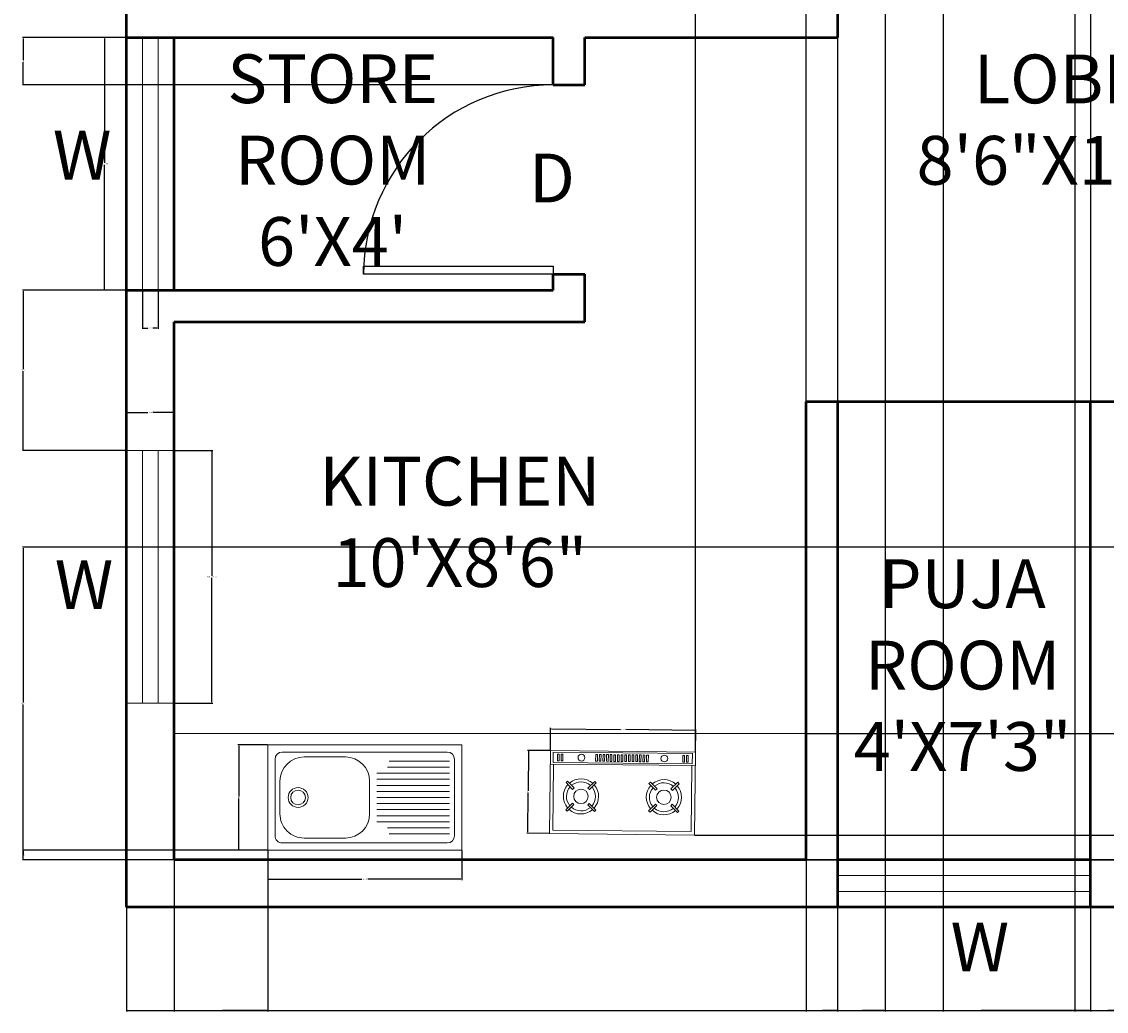
# Model space of a CAD drawing. Units: inches. Extents: x 1916 to 2328, y 785 to 1125.
# Tile 1 of 3: x 1916 to 2122, y 785 to 973. Entities that reach past the tile are written whole.
import ezdxf

# ---------------------------------------------------------------- set-up
doc = ezdxf.new("R2010")
doc.units = ezdxf.units.IN
for name, color, linetype, lineweight in [('A-ANNO-DIMS', 2, 'Continuous', 18), ('A-ANNO-TEXT', 7, 'Continuous', 18), ('A-AREA-IDEN', 7, 'Continuous', 25), ('A-DOOR', 3, 'Continuous', 25), ('A-EQPM', 8, 'Continuous', 18), ('A-FLOR-FIXT', 9, 'Continuous', 18), ('A-GLAZ', 4, 'Continuous', 18), ('A-WALL', 7, 'Continuous', 50)]:
    doc.layers.add(name, color=color, linetype=linetype, lineweight=lineweight)
doc.styles.get("Standard").update_dxf_attribs({"font": 'arial.ttf'})
doc.dimstyles.get("Standard").update_dxf_attribs({"dimtxt": 0.18, "dimasz": 0.18, "dimexe": 0.18, "dimexo": 0.0625, "dimgap": 0.09, "dimtad": 0, "dimtih": 1, "dimtoh": 1, "dimdec": 4, "dimzin": 0, "dimdsep": 46, "dimtxsty": 'Standard', "dimcen": 0.09, "dimadec": 0, "dimazin": 0, "dimtfac": 1, "dimtdec": 4, "dimtofl": 0, "dimtmove": 0, "dimatfit": 3, "dimfxl": 1, "dimtolj": 1, "dimtzin": 0, "dimarcsym": 0})

# ---------------------------------------------------------------- blocks, each defined once
blk = doc.blocks.new('*U2')
for p, q in [((0, 0), (0, -6)), ((40, 0), (40, -6))]:
    blk.add_line(p, q)
blk.add_lwpolyline([(0, 0), (0, 40), (1.75, 40), (1.75, 0)], close=True)
blk.add_arc((0, 0), 40, 0, 90)
blk = doc.blocks.new('A$C56104318')
for p, q in [((0, 0.609), (1.12, 0.609)), ((0, 0.609), (0, 0)), ((0.084, 0.567), (1.036, 0.567)), ((1.12, 0.609), (1.12, 0)), ((0.042, 0.525), (0.042, 0.084)), ((0.42, 0.5145), (0.07, 0.5145)), ((0.672, 0.539), (0.91, 0.539)), ((1.078, 0.525), (1.078, 0.084)), ((0.07, 0.4795), (0.4294, 0.4795)), ((0.07, 0.4445), (0.49, 0.4445)), ((0.07, 0.4095), (0.49, 0.4095)), ((0.532, 0.21), (0.532, 0.399)), ((1.05, 0.399), (1.05, 0.21)), ((0.07, 0.3745), (0.49, 0.3745)), ((0.07, 0.3395), (0.49, 0.3395)), ((0.07, 0.3045), (0.49, 0.3045)), ((0.07, 0.2695), (0.49, 0.2695)), ((0.07, 0.2345), (0.49, 0.2345)), ((0.07, 0.1995), (0.49, 0.1995)), ((0.07, 0.1645), (0.4898, 0.1645)), ((0.07, 0.1295), (0.4294, 0.1295)), ((0.07, 0.0945), (0.42, 0.0945)), ((0.91, 0.07), (0.672, 0.07)), ((1.036, 0.042), (0.084, 0.042)), ((1.12, 0), (0, 0))]:
    blk.add_line(p, q)
for radius in [0.0574, 0.0427]:
    blk.add_circle((0.945, 0.3045), radius)
for centre, radius, start, end in [((0.084, 0.525), 0.042, 90, 180), ((1.036, 0.525), 0.042, 0, 90), ((0.672, 0.399), 0.14, 90, 180), ((0.91, 0.399), 0.14, 0, 90), ((0.672, 0.21), 0.14, 180, 270), ((0.91, 0.21), 0.14, 270, 0.00001), ((0.084, 0.084), 0.042, 180, 270), ((1.036, 0.084), 0.042, 270, 0.00001)]:
    blk.add_arc(centre, radius, start, end)
blk = doc.blocks.new('A$C7812624E')
for p, q in [((0, 399.8), (700, 399.8)), ((0, 399.8), (0, 0)), ((16.5, 383.3), (683.5, 383.3)), ((16.5, 383.3), (16.5, 64.8)), ((683.5, 383.3), (683.5, 64.8)), ((700, 399.8), (700, 0)), ((84.4, 292.2), (77.3, 285.1)), ((77.3, 285.1), (109.7, 252.7)), ((84.4, 292.2), (116.8, 259.8)), ((215.8, 292), (183.4, 259.6)), ((222.9, 284.9), (190.5, 252.5)), ((222.9, 284.9), (215.8, 292)), ((484.4, 292.2), (477.3, 285.1)), ((477.3, 285.1), (509.7, 252.7)), ((484.4, 292.2), (516.8, 259.8)), ((615.8, 292), (583.4, 259.6)), ((622.9, 284.9), (590.5, 252.5)), ((622.9, 284.9), (615.8, 292)), ((116.8, 259.8), (109.7, 252.7)), ((190.5, 252.5), (183.4, 259.6)), ((516.8, 259.8), (509.7, 252.7)), ((590.5, 252.5), (583.4, 259.6)), ((77.3, 153.5), (109.7, 185.9)), ((84.4, 146.5), (116.8, 178.8)), ((116.8, 178.8), (109.7, 185.9)), ((190.5, 186.1), (183.4, 179)), ((215.8, 146.6), (183.4, 179)), ((222.9, 153.7), (190.5, 186.1)), ((477.3, 153.5), (509.7, 185.9)), ((484.4, 146.5), (516.8, 178.8)), ((516.8, 178.8), (509.7, 185.9)), ((590.5, 186.1), (583.4, 179)), ((615.8, 146.6), (583.4, 179)), ((622.9, 153.7), (590.5, 186.1)), ((84.4, 146.5), (77.3, 153.5)), ((222.9, 153.7), (215.8, 146.6)), ((484.4, 146.5), (477.3, 153.5)), ((622.9, 153.7), (615.8, 146.6)), ((0, 64.8), (700, 64.8)), ((15, 56.8), (15, 7.3)), ((686.4, 56.8), (15, 56.8)), ((686.4, 7.3), (686.4, 56.8)), ((15, 7.3), (686.4, 7.3)), ((42.8, 48.8), (34.7, 48.8)), ((34.7, 48.8), (34.7, 16.4)), ((34.7, 16.4), (42.8, 16.4)), ((42.8, 16.4), (42.8, 48.8)), ((60.4, 48.8), (52.3, 48.8)), ((52.3, 48.8), (52.3, 16.4)), ((52.3, 16.4), (60.4, 16.4)), ((60.4, 16.4), (60.4, 48.8)), ((235.4, 48.8), (227.3, 48.8)), ((227.3, 48.8), (227.3, 16.4)), ((227.3, 16.4), (235.4, 16.4)), ((235.4, 16.4), (235.4, 48.8)), ((252.9, 48.8), (244.8, 48.8)), ((244.8, 48.8), (244.8, 16.4)), ((244.8, 16.4), (252.9, 16.4)), ((252.9, 16.4), (252.9, 48.8)), ((270.5, 48.8), (262.4, 48.8)), ((262.4, 48.8), (262.4, 16.4)), ((262.4, 16.4), (270.5, 16.4)), ((270.5, 16.4), (270.5, 48.8)), ((288, 48.8), (279.9, 48.8)), ((279.9, 48.8), (279.9, 16.4)), ((279.9, 16.4), (288, 16.4)), ((288, 16.4), (288, 48.8)), ((305.5, 48.8), (297.5, 48.8)), ((297.5, 48.8), (297.5, 16.4)), ((297.5, 16.4), (305.5, 16.4)), ((305.5, 16.4), (305.5, 48.8)), ((323.1, 48.8), (315, 48.8)), ((315, 48.8), (315, 16.4)), ((315, 16.4), (323.1, 16.4)), ((323.1, 16.4), (323.1, 48.8)), ((340.6, 48.8), (332.5, 48.8)), ((332.5, 48.8), (332.5, 16.4)), ((332.5, 16.4), (340.6, 16.4)), ((340.6, 16.4), (340.6, 48.8)), ((358.2, 48.8), (350.1, 48.8)), ((350.1, 48.8), (350.1, 16.4)), ((350.1, 16.4), (358.2, 16.4)), ((358.2, 16.4), (358.2, 48.8)), ((375.7, 48.8), (367.6, 48.8)), ((367.6, 48.8), (367.6, 16.4)), ((367.6, 16.4), (375.7, 16.4)), ((375.7, 16.4), (375.7, 48.8)), ((393.3, 48.8), (385.2, 48.8)), ((385.2, 48.8), (385.2, 16.4)), ((385.2, 16.4), (393.3, 16.4)), ((393.3, 16.4), (393.3, 48.8)), ((410.8, 48.8), (402.7, 48.8)), ((402.7, 48.8), (402.7, 16.4)), ((402.7, 16.4), (410.8, 16.4)), ((410.8, 16.4), (410.8, 48.8)), ((428.3, 48.8), (420.2, 48.8)), ((420.2, 48.8), (420.2, 16.4)), ((420.2, 16.4), (428.3, 16.4)), ((428.3, 16.4), (428.3, 48.8)), ((445.9, 48.8), (437.8, 48.8)), ((437.8, 48.8), (437.8, 16.4)), ((437.8, 16.4), (445.9, 16.4)), ((445.9, 16.4), (445.9, 48.8)), ((463.4, 48.8), (455.3, 48.8)), ((455.3, 48.8), (455.3, 16.4)), ((455.3, 16.4), (463.4, 16.4)), ((463.4, 16.4), (463.4, 48.8)), ((481, 48.8), (472.9, 48.8)), ((472.9, 48.8), (472.9, 16.4)), ((472.9, 16.4), (481, 16.4)), ((481, 16.4), (481, 48.8)), ((639.6, 16.4), (639.6, 48.8)), ((639.6, 48.8), (647.7, 48.8)), ((647.7, 16.4), (639.6, 16.4)), ((647.7, 48.8), (647.7, 16.4)), ((657.2, 16.4), (657.2, 48.8)), ((657.2, 48.8), (665.3, 48.8)), ((665.3, 16.4), (657.2, 16.4)), ((665.3, 48.8), (665.3, 16.4)), ((0, 0), (700, 0))]:
    blk.add_line(p, q)
for centre, radius in [((150, 219.3), 35), ((550, 219.3), 35), ((150, 32.3), 16.3), ((550, 32.3), 16.3)]:
    blk.add_circle(centre, radius)
for centre, radius, start, end in [((150, 219.3), 85, 138.279, 221.721), ((150, 219.3), 70, 138.9827, 221.0173), ((150, 219.3), 85, 48.279, 131.5344), ((150, 219.3), 70, 48.9827, 130.7906), ((150, 219.3), 70, 319.2094, 40.7906), ((150, 219.3), 85, 318.4656, 41.5344), ((550, 219.3), 85, 138.279, 221.721), ((550, 219.3), 70, 138.9827, 221.0173), ((550, 219.3), 85, 48.279, 131.5344), ((550, 219.3), 70, 48.9827, 130.7906), ((550, 219.3), 70, 319.2094, 40.7906), ((550, 219.3), 85, 318.4656, 41.5344), ((150, 219.3), 70, 229.2094, 311.0173), ((550, 219.3), 70, 229.2094, 311.0173), ((150, 219.3), 85, 228.4656, 311.721), ((550, 219.3), 85, 228.4656, 311.721)]:
    blk.add_arc(centre, radius, start, end)
blk = doc.blocks.new('WIN-48-JAMB-9')
for p, q in [((0, 9), (0, 0)), ((48, 9), (48, 0)), ((48, 6), (0, 6)), ((48, 3), (0, 3))]:
    blk.add_line(p, q)
blk = doc.blocks.new('WIN-48-SASH')
for p, q in [((48, 3), (0, 3)), ((48, 0), (0, 0))]:
    blk.add_line(p, q)
blk = doc.blocks.new('*D15')
at = {"layer": 'A-ANNO-DIMS', "color": 0, "lineweight": -2, "transparency": 16777216}
for p, q in [((1945.3, 891.65), (1952.61, 891.65)), ((1952.43, 891.47), (1952.43, 867.83)), ((1952.43, 843.83), (1952.43, 867.47)), ((1945.3, 843.65), (1952.61, 843.65))]:
    blk.add_line(p, q, dxfattribs=at)
at = {"layer": 'A-ANNO-DIMS', "color": 0, "transparency": 16777216}
for points in [[(1952.4, 891.47), (1952.46, 891.47), (1952.43, 891.65)], [(1952.4, 843.83), (1952.46, 843.83), (1952.43, 843.65)]]:
    blk.add_solid(points, dxfattribs=at)
at = {"layer": 'Defpoints', "color": 0, "transparency": 16777216}
for p in [(1945.23, 891.65), (1952.43, 891.65), (1945.23, 843.65)]:
    blk.add_point(p, dxfattribs=at)
at = {"layer": 'A-ANNO-DIMS', "color": 0, "transparency": 16777216, "insert": (1952.43, 867.65), "char_height": 0.18, "attachment_point": 5}
blk.add_mtext('\\A1;WINDOW 48 TYP.', dxfattribs=at)
blk = doc.blocks.new('*D16')
at = {"layer": 'A-ANNO-DIMS', "color": 0, "lineweight": -2, "transparency": 16777216}
for p, q in [((1936.23, 891.71), (1936.23, 899.03)), ((1936.41, 898.85), (1940.28, 898.85)), ((1945.05, 898.85), (1941.19, 898.85)), ((1945.23, 891.71), (1945.23, 899.03))]:
    blk.add_line(p, q, dxfattribs=at)
at = {"layer": 'A-ANNO-DIMS', "color": 0, "transparency": 16777216}
for points in [[(1936.41, 898.88), (1936.41, 898.82), (1936.23, 898.85)], [(1945.05, 898.88), (1945.05, 898.82), (1945.23, 898.85)]]:
    blk.add_solid(points, dxfattribs=at)
at = {"layer": 'Defpoints', "color": 0, "transparency": 16777216}
for p in [(1936.23, 898.85), (1936.23, 891.65), (1945.23, 891.65)]:
    blk.add_point(p, dxfattribs=at)
at = {"layer": 'A-ANNO-DIMS', "color": 0, "transparency": 16777216, "insert": (1940.73, 898.85), "char_height": 0.18, "attachment_point": 5}
blk.add_mtext('\\A1;9 TYP.', dxfattribs=at)
blk = doc.blocks.new('*D23')
at = {"layer": 'A-ANNO-DIMS', "color": 0, "lineweight": -2, "transparency": 16777216}
for p, q in [((1939.17, 970.1), (1931.85, 970.1)), ((1932.03, 969.92), (1932.03, 946.28)), ((1932.03, 922.28), (1932.03, 945.92)), ((1939.17, 922.1), (1931.85, 922.1))]:
    blk.add_line(p, q, dxfattribs=at)
at = {"layer": 'A-ANNO-DIMS', "color": 0, "transparency": 16777216}
for points in [[(1932, 969.92), (1932.06, 969.92), (1932.03, 970.1)], [(1932, 922.28), (1932.06, 922.28), (1932.03, 922.1)]]:
    blk.add_solid(points, dxfattribs=at)
at = {"layer": 'Defpoints', "color": 0, "transparency": 16777216}
for p in [(1939.23, 970.1), (1932.03, 922.1), (1939.23, 922.1)]:
    blk.add_point(p, dxfattribs=at)
at = {"layer": 'A-ANNO-DIMS', "color": 0, "transparency": 16777216, "insert": (1932.03, 946.1), "char_height": 0.18, "attachment_point": 5}
blk.add_mtext('\\A1;SASH 48 TYP.', dxfattribs=at)
blk = doc.blocks.new('*D24')
at = {"layer": 'A-ANNO-DIMS', "color": 0, "lineweight": -2, "transparency": 16777216}
for p, q in [((1939.23, 922.04), (1939.23, 914.72)), ((1942.23, 922.04), (1942.23, 914.72)), ((1939.41, 914.9), (1940.28, 914.9)), ((1942.05, 914.9), (1941.19, 914.9))]:
    blk.add_line(p, q, dxfattribs=at)
at = {"layer": 'A-ANNO-DIMS', "color": 0, "transparency": 16777216}
for points in [[(1939.41, 914.93), (1939.41, 914.87), (1939.23, 914.9)], [(1942.05, 914.93), (1942.05, 914.87), (1942.23, 914.9)]]:
    blk.add_solid(points, dxfattribs=at)
at = {"layer": 'Defpoints', "color": 0, "transparency": 16777216}
for p in [(1939.23, 922.1), (1942.23, 922.1), (1942.23, 914.9)]:
    blk.add_point(p, dxfattribs=at)
at = {"layer": 'A-ANNO-DIMS', "color": 0, "transparency": 16777216, "insert": (1940.73, 914.9), "char_height": 0.18, "attachment_point": 5}
blk.add_mtext('\\A1;3 TYP.', dxfattribs=at)
blk = doc.blocks.new('*D25')
at = {"layer": 'A-ANNO-DIMS', "color": 0, "lineweight": -2, "transparency": 16777216}
for p, q in [((1963.03, 815.63), (1963.03, 809.99)), ((1999.87, 815.63), (1999.87, 809.99)), ((1963.21, 810.17), (1980.9, 810.17)), ((1999.69, 810.17), (1982, 810.17))]:
    blk.add_line(p, q, dxfattribs=at)
at = {"layer": 'A-ANNO-DIMS', "color": 0, "transparency": 16777216}
for points in [[(1963.21, 810.2), (1963.21, 810.14), (1963.03, 810.17)], [(1999.69, 810.2), (1999.69, 810.14), (1999.87, 810.17)]]:
    blk.add_solid(points, dxfattribs=at)
at = {"layer": 'Defpoints', "color": 0, "transparency": 16777216}
for p in [(1963.03, 815.69), (1999.87, 815.69), (1963.03, 810.17)]:
    blk.add_point(p, dxfattribs=at)
at = {"layer": 'A-ANNO-DIMS', "color": 0, "transparency": 16777216, "insert": (1981.45, 810.17), "char_height": 0.18, "attachment_point": 5}
blk.add_mtext('\\A1;SINK 37', dxfattribs=at)
blk = doc.blocks.new('*D26')
at = {"layer": 'A-ANNO-DIMS', "color": 0, "lineweight": -2, "transparency": 16777216}
for p, q in [((1962.97, 835.72), (1957.33, 835.72)), ((1957.51, 835.54), (1957.51, 825.89)), ((1957.51, 815.87), (1957.51, 825.52)), ((1962.97, 815.69), (1957.33, 815.69))]:
    blk.add_line(p, q, dxfattribs=at)
at = {"layer": 'A-ANNO-DIMS', "color": 0, "transparency": 16777216}
for points in [[(1957.48, 835.54), (1957.54, 835.54), (1957.51, 835.72)], [(1957.48, 815.87), (1957.54, 815.87), (1957.51, 815.69)]]:
    blk.add_solid(points, dxfattribs=at)
at = {"layer": 'Defpoints', "color": 0, "transparency": 16777216}
for p in [(1957.51, 835.72), (1963.03, 835.72), (1963.03, 815.69)]:
    blk.add_point(p, dxfattribs=at)
at = {"layer": 'A-ANNO-DIMS', "color": 0, "transparency": 16777216, "insert": (1957.51, 825.71), "char_height": 0.18, "attachment_point": 5}
blk.add_mtext('\\A1;20', dxfattribs=at)
blk = doc.blocks.new('*D27')
at = {"layer": 'A-ANNO-DIMS', "color": 0, "lineweight": -2, "transparency": 16777216}
for p, q in [((2016.68, 834.68), (2016.73, 838.93)), ((2016.91, 838.75), (2029.99, 838.61)), ((2044.11, 838.46), (2031.03, 838.6)), ((2044.24, 834.38), (2044.29, 838.63))]:
    blk.add_line(p, q, dxfattribs=at)
at = {"layer": 'A-ANNO-DIMS', "color": 0, "transparency": 16777216}
for points in [[(2016.91, 838.78), (2016.91, 838.72), (2016.73, 838.75)], [(2044.11, 838.49), (2044.11, 838.43), (2044.29, 838.45)]]:
    blk.add_solid(points, dxfattribs=at)
at = {"layer": 'Defpoints', "color": 0, "transparency": 16777216}
for p in [(2016.73, 838.75), (2016.68, 834.62), (2044.24, 834.32)]:
    blk.add_point(p, dxfattribs=at)
at = {"layer": 'A-ANNO-DIMS', "color": 0, "transparency": 16777216, "insert": (2030.51, 838.6), "char_height": 0.18, "attachment_point": 5}
blk.add_mtext('\\A1;HOB 28', dxfattribs=at)
blk = doc.blocks.new('*D28')
at = {"layer": 'A-ANNO-DIMS', "color": 0, "lineweight": -2, "transparency": 16777216}
for p, q in [((2016.62, 834.62), (2012.37, 834.66)), ((2012.55, 834.48), (2012.47, 826.97)), ((2012.38, 819.1), (2012.46, 826.61)), ((2016.45, 818.88), (2012.2, 818.92))]:
    blk.add_line(p, q, dxfattribs=at)
at = {"layer": 'A-ANNO-DIMS', "color": 0, "transparency": 16777216}
for points in [[(2012.52, 834.48), (2012.58, 834.48), (2012.55, 834.66)], [(2012.35, 819.1), (2012.41, 819.1), (2012.38, 818.92)]]:
    blk.add_solid(points, dxfattribs=at)
at = {"layer": 'Defpoints', "color": 0, "transparency": 16777216}
for p in [(2016.68, 834.62), (2012.38, 818.92), (2016.51, 818.88)]:
    blk.add_point(p, dxfattribs=at)
at = {"layer": 'A-ANNO-DIMS', "color": 0, "transparency": 16777216, "insert": (2012.47, 826.79), "char_height": 0.18, "attachment_point": 5}
blk.add_mtext('\\A1;16', dxfattribs=at)
blk = doc.blocks.new('*D35')
at = {"layer": 'A-ANNO-DIMS', "color": 0, "lineweight": -2, "transparency": 16777216}
for p, q in [((1936.17, 922.1), (1916.44, 922.1)), ((1916.62, 921.92), (1916.62, 907.06)), ((1916.62, 891.83), (1916.62, 906.69)), ((1936.17, 891.65), (1916.44, 891.65))]:
    blk.add_line(p, q, dxfattribs=at)
at = {"layer": 'A-ANNO-DIMS', "color": 0, "transparency": 16777216}
for points in [[(1916.59, 921.92), (1916.65, 921.92), (1916.62, 922.1)], [(1916.59, 891.83), (1916.65, 891.83), (1916.62, 891.65)]]:
    blk.add_solid(points, dxfattribs=at)
at = {"layer": 'Defpoints', "color": 0, "transparency": 16777216}
for p in [(1916.62, 922.1), (1936.23, 922.1), (1936.23, 891.65)]:
    blk.add_point(p, dxfattribs=at)
at = {"layer": 'A-ANNO-DIMS', "color": 0, "transparency": 16777216, "insert": (1916.62, 906.88), "char_height": 0.18, "attachment_point": 5}
blk.add_mtext('\\A1;30.45', dxfattribs=at)
blk = doc.blocks.new('*D36')
at = {"layer": 'A-ANNO-DIMS', "color": 0, "lineweight": -2, "transparency": 16777216}
for p, q in [((2299.17, 873.26), (1916.44, 873.26)), ((1916.62, 873.08), (1916.62, 843.75)), ((1916.62, 814.06), (1916.62, 843.39)), ((2299.17, 813.88), (1916.44, 813.88))]:
    blk.add_line(p, q, dxfattribs=at)
at = {"layer": 'A-ANNO-DIMS', "color": 0, "transparency": 16777216}
for points in [[(1916.59, 873.08), (1916.65, 873.08), (1916.62, 873.26)], [(1916.59, 814.06), (1916.65, 814.06), (1916.62, 813.88)]]:
    blk.add_solid(points, dxfattribs=at)
at = {"layer": 'Defpoints', "color": 0, "transparency": 16777216}
for p in [(1916.62, 873.26), (2299.23, 873.26), (2299.23, 813.88)]:
    blk.add_point(p, dxfattribs=at)
at = {"layer": 'A-ANNO-DIMS', "color": 0, "transparency": 16777216, "insert": (1916.62, 843.57), "char_height": 0.18, "attachment_point": 5}
blk.add_mtext('\\A1;59.38', dxfattribs=at)
blk = doc.blocks.new('*D37')
at = {"layer": 'A-ANNO-DIMS', "color": 0, "lineweight": -2, "transparency": 16777216}
for p, q in [((2119.23, 804.82), (2119.23, 785.08)), ((2131.87, 804.82), (2131.87, 785.08)), ((2119.41, 785.26), (2125.1, 785.26)), ((2131.69, 785.26), (2126.01, 785.26))]:
    blk.add_line(p, q, dxfattribs=at)
at = {"layer": 'A-ANNO-DIMS', "color": 0, "transparency": 16777216}
for points in [[(2119.41, 785.29), (2119.41, 785.23), (2119.23, 785.26)], [(2131.69, 785.29), (2131.69, 785.23), (2131.87, 785.26)]]:
    blk.add_solid(points, dxfattribs=at)
at = {"layer": 'Defpoints', "color": 0, "transparency": 16777216}
for p in [(2119.23, 804.88), (2131.87, 804.88), (2131.87, 785.26)]:
    blk.add_point(p, dxfattribs=at)
at = {"layer": 'A-ANNO-DIMS', "color": 0, "transparency": 16777216, "insert": (2125.55, 785.26), "char_height": 0.18, "attachment_point": 5}
blk.add_mtext('\\A1;12.642', dxfattribs=at)
blk = doc.blocks.new('*D40')
at = {"layer": 'A-ANNO-DIMS', "color": 0, "lineweight": -2, "transparency": 16777216}
for p, q in [((2065.23, 813.82), (2065.23, 785.08)), ((2071.23, 804.82), (2071.23, 785.08)), ((2065.41, 785.26), (2068.08, 785.26)), ((2071.05, 785.26), (2068.38, 785.26))]:
    blk.add_line(p, q, dxfattribs=at)
at = {"layer": 'A-ANNO-DIMS', "color": 0, "transparency": 16777216}
for points in [[(2065.41, 785.29), (2065.41, 785.23), (2065.23, 785.26)], [(2071.05, 785.29), (2071.05, 785.23), (2071.23, 785.26)]]:
    blk.add_solid(points, dxfattribs=at)
at = {"layer": 'Defpoints', "color": 0, "transparency": 16777216}
for p in [(2065.23, 813.88), (2071.23, 804.88), (2071.23, 785.26)]:
    blk.add_point(p, dxfattribs=at)
at = {"layer": 'A-ANNO-DIMS', "color": 0, "transparency": 16777216, "insert": (2068.23, 785.26), "char_height": 0.18, "attachment_point": 5}
blk.add_mtext('\\A1;6', dxfattribs=at)
blk = doc.blocks.new('*D41')
at = {"layer": 'A-ANNO-DIMS', "color": 0, "lineweight": -2, "transparency": 16777216}
for p, q in [((2065.3, 837.88), (2328.03, 837.88)), ((2327.85, 837.7), (2327.85, 826.06)), ((2327.85, 814.06), (2327.85, 825.7)), ((2065.3, 813.88), (2328.03, 813.88))]:
    blk.add_line(p, q, dxfattribs=at)
at = {"layer": 'A-ANNO-DIMS', "color": 0, "transparency": 16777216}
for points in [[(2327.82, 837.7), (2327.88, 837.7), (2327.85, 837.88)], [(2327.82, 814.06), (2327.88, 814.06), (2327.85, 813.88)]]:
    blk.add_solid(points, dxfattribs=at)
at = {"layer": 'Defpoints', "color": 0, "transparency": 16777216}
for p in [(2065.23, 837.88), (2327.85, 837.88), (2065.23, 813.88)]:
    blk.add_point(p, dxfattribs=at)
at = {"layer": 'A-ANNO-DIMS', "color": 0, "transparency": 16777216, "insert": (2327.85, 825.88), "char_height": 0.18, "attachment_point": 5}
blk.add_mtext('\\A1;24', dxfattribs=at)
blk = doc.blocks.new('*D42')
at = {"layer": 'A-ANNO-DIMS', "color": 0, "lineweight": -2, "transparency": 16777216}
for p, q in [((1963.03, 815.63), (1963.03, 785.08)), ((1945.23, 813.82), (1945.23, 785.08)), ((1945.41, 785.26), (1953.82, 785.26)), ((1962.85, 785.26), (1954.45, 785.26))]:
    blk.add_line(p, q, dxfattribs=at)
at = {"layer": 'A-ANNO-DIMS', "color": 0, "transparency": 16777216}
for points in [[(1945.41, 785.29), (1945.41, 785.23), (1945.23, 785.26)], [(1962.85, 785.29), (1962.85, 785.23), (1963.03, 785.26)]]:
    blk.add_solid(points, dxfattribs=at)
at = {"layer": 'Defpoints', "color": 0, "transparency": 16777216}
for p in [(1963.03, 815.69), (1945.23, 813.88), (1963.03, 785.26)]:
    blk.add_point(p, dxfattribs=at)
at = {"layer": 'A-ANNO-DIMS', "color": 0, "transparency": 16777216, "insert": (1954.13, 785.26), "char_height": 0.18, "attachment_point": 5}
blk.add_mtext('\\A1;17.8', dxfattribs=at)
blk = doc.blocks.new('*D43')
at = {"layer": 'A-ANNO-DIMS', "color": 0, "lineweight": -2, "transparency": 16777216}
for p, q in [((2044.24, 834.38), (2044.24, 1124.67)), ((2044.42, 1124.49), (2054.27, 1124.49)), ((2065.05, 1124.49), (2055.2, 1124.49)), ((2065.23, 837.94), (2065.23, 1124.67))]:
    blk.add_line(p, q, dxfattribs=at)
at = {"layer": 'A-ANNO-DIMS', "color": 0, "transparency": 16777216}
for points in [[(2044.42, 1124.52), (2044.42, 1124.46), (2044.24, 1124.49)], [(2065.05, 1124.52), (2065.05, 1124.46), (2065.23, 1124.49)]]:
    blk.add_solid(points, dxfattribs=at)
at = {"layer": 'Defpoints', "color": 0, "transparency": 16777216}
for p in [(2065.23, 1124.49), (2065.23, 837.88), (2044.24, 834.32)]:
    blk.add_point(p, dxfattribs=at)
at = {"layer": 'A-ANNO-DIMS', "color": 0, "transparency": 16777216, "insert": (2054.74, 1124.49), "char_height": 0.18, "attachment_point": 5}
blk.add_mtext('\\A1;20.992', dxfattribs=at)
blk = doc.blocks.new('*D44')
at = {"layer": 'A-ANNO-DIMS', "color": 0, "lineweight": -2, "transparency": 16777216}
for p, q in [((1962.97, 815.69), (1916.44, 815.69)), ((1916.62, 815.51), (1916.62, 814.97)), ((1945.17, 813.88), (1916.44, 813.88)), ((1916.62, 814.06), (1916.62, 814.6))]:
    blk.add_line(p, q, dxfattribs=at)
at = {"layer": 'A-ANNO-DIMS', "color": 0, "transparency": 16777216}
for points in [[(1916.59, 815.51), (1916.65, 815.51), (1916.62, 815.69)], [(1916.59, 814.06), (1916.65, 814.06), (1916.62, 813.88)]]:
    blk.add_solid(points, dxfattribs=at)
at = {"layer": 'Defpoints', "color": 0, "transparency": 16777216}
for p in [(1963.03, 815.69), (1916.62, 813.88), (1945.23, 813.88)]:
    blk.add_point(p, dxfattribs=at)
at = {"layer": 'A-ANNO-DIMS', "color": 0, "transparency": 16777216, "insert": (1916.62, 814.79), "char_height": 0.18, "attachment_point": 5}
blk.add_mtext('\\A1;1.812', dxfattribs=at)
blk = doc.blocks.new('*D45')
at = {"layer": 'A-ANNO-DIMS', "color": 0, "lineweight": -2, "transparency": 16777216}
for p, q in [((2044.13, 818.58), (2328.03, 818.58)), ((2327.85, 818.4), (2327.85, 816.41)), ((2327.85, 814.06), (2327.85, 816.05)), ((2065.3, 813.88), (2328.03, 813.88))]:
    blk.add_line(p, q, dxfattribs=at)
at = {"layer": 'A-ANNO-DIMS', "color": 0, "transparency": 16777216}
for points in [[(2327.82, 818.4), (2327.88, 818.4), (2327.85, 818.58)], [(2327.82, 814.06), (2327.88, 814.06), (2327.85, 813.88)]]:
    blk.add_solid(points, dxfattribs=at)
at = {"layer": 'Defpoints', "color": 0, "transparency": 16777216}
for p in [(2044.07, 818.58), (2065.23, 813.88), (2327.85, 813.88)]:
    blk.add_point(p, dxfattribs=at)
at = {"layer": 'A-ANNO-DIMS', "color": 0, "transparency": 16777216, "insert": (2327.85, 816.23), "char_height": 0.18, "attachment_point": 5}
blk.add_mtext('\\A1;4.702', dxfattribs=at)
blk = doc.blocks.new('*D47')
at = {"layer": 'A-ANNO-DIMS', "color": 0, "lineweight": -2, "transparency": 16777216}
for p, q in [((2091.23, 1077.66), (2091.23, 785.08)), ((2119.23, 1067.16), (2119.23, 785.08)), ((2091.41, 785.26), (2105.01, 785.26)), ((2119.05, 785.26), (2105.45, 785.26))]:
    blk.add_line(p, q, dxfattribs=at)
at = {"layer": 'A-ANNO-DIMS', "color": 0, "transparency": 16777216}
for points in [[(2091.41, 785.29), (2091.41, 785.23), (2091.23, 785.26)], [(2119.05, 785.29), (2119.05, 785.23), (2119.23, 785.26)]]:
    blk.add_solid(points, dxfattribs=at)
at = {"layer": 'Defpoints', "color": 0, "transparency": 16777216}
for p in [(2091.23, 1077.72), (2119.23, 1067.22), (2119.23, 785.26)]:
    blk.add_point(p, dxfattribs=at)
at = {"layer": 'A-ANNO-DIMS', "color": 0, "transparency": 16777216, "insert": (2105.23, 785.26), "char_height": 0.18, "attachment_point": 5}
blk.add_mtext('\\A1;28', dxfattribs=at)
blk = doc.blocks.new('*D50')
at = {"layer": 'A-ANNO-DIMS', "color": 0, "lineweight": -2, "transparency": 16777216}
for p, q in [((2071.23, 1024.04), (2071.23, 785.08)), ((2080.23, 1024.04), (2080.23, 785.08)), ((2071.41, 785.26), (2075.58, 785.26)), ((2080.05, 785.26), (2075.88, 785.26))]:
    blk.add_line(p, q, dxfattribs=at)
at = {"layer": 'A-ANNO-DIMS', "color": 0, "transparency": 16777216}
for points in [[(2071.41, 785.29), (2071.41, 785.23), (2071.23, 785.26)], [(2080.05, 785.29), (2080.05, 785.23), (2080.23, 785.26)]]:
    blk.add_solid(points, dxfattribs=at)
at = {"layer": 'Defpoints', "color": 0, "transparency": 16777216}
for p in [(2071.23, 1024.1), (2080.23, 1024.1), (2080.23, 785.26)]:
    blk.add_point(p, dxfattribs=at)
at = {"layer": 'A-ANNO-DIMS', "color": 0, "transparency": 16777216, "insert": (2075.73, 785.26), "char_height": 0.18, "attachment_point": 5}
blk.add_mtext('\\A1;9', dxfattribs=at)
blk = doc.blocks.new('*D51')
at = {"layer": 'A-ANNO-DIMS', "color": 0, "lineweight": -2, "transparency": 16777216}
for p, q in [((2080.23, 1024.04), (2080.23, 785.08)), ((2116.23, 1024.04), (2116.23, 785.08)), ((2080.41, 785.26), (2098.01, 785.26)), ((2116.05, 785.26), (2098.45, 785.26))]:
    blk.add_line(p, q, dxfattribs=at)
at = {"layer": 'A-ANNO-DIMS', "color": 0, "transparency": 16777216}
for points in [[(2080.41, 785.29), (2080.41, 785.23), (2080.23, 785.26)], [(2116.05, 785.29), (2116.05, 785.23), (2116.23, 785.26)]]:
    blk.add_solid(points, dxfattribs=at)
at = {"layer": 'Defpoints', "color": 0, "transparency": 16777216}
for p in [(2080.23, 1024.1), (2116.23, 1024.1), (2116.23, 785.26)]:
    blk.add_point(p, dxfattribs=at)
at = {"layer": 'A-ANNO-DIMS', "color": 0, "transparency": 16777216, "insert": (2098.23, 785.26), "char_height": 0.18, "attachment_point": 5}
blk.add_mtext('\\A1;36', dxfattribs=at)
blk = doc.blocks.new('*D53')
at = {"layer": 'A-ANNO-DIMS', "color": 0, "lineweight": -2, "transparency": 16777216}
for p, q in [((2017.17, 970.1), (1916.44, 970.1)), ((1916.62, 969.92), (1916.62, 965.78)), ((1916.62, 961.28), (1916.62, 965.42)), ((2017.17, 961.1), (1916.44, 961.1))]:
    blk.add_line(p, q, dxfattribs=at)
at = {"layer": 'A-ANNO-DIMS', "color": 0, "transparency": 16777216}
for points in [[(1916.59, 969.92), (1916.65, 969.92), (1916.62, 970.1)], [(1916.59, 961.28), (1916.65, 961.28), (1916.62, 961.1)]]:
    blk.add_solid(points, dxfattribs=at)
at = {"layer": 'Defpoints', "color": 0, "transparency": 16777216}
for p in [(1916.62, 970.1), (2017.23, 970.1), (2017.23, 961.1)]:
    blk.add_point(p, dxfattribs=at)
at = {"layer": 'A-ANNO-DIMS', "color": 0, "transparency": 16777216, "insert": (1916.62, 965.6), "char_height": 0.18, "attachment_point": 5}
blk.add_mtext('\\A1;9', dxfattribs=at)
blk = doc.blocks.new('*D57')
at = {"layer": 'A-ANNO-DIMS', "color": 0, "lineweight": -2, "transparency": 16777216}
for p, q in [((1936.23, 804.82), (1936.23, 785.08)), ((2308.23, 804.82), (2308.23, 785.08)), ((1936.41, 785.26), (2121.95, 785.26)), ((2308.05, 785.26), (2122.52, 785.26))]:
    blk.add_line(p, q, dxfattribs=at)
at = {"layer": 'A-ANNO-DIMS', "color": 0, "transparency": 16777216}
for points in [[(1936.41, 785.29), (1936.41, 785.23), (1936.23, 785.26)], [(2308.05, 785.29), (2308.05, 785.23), (2308.23, 785.26)]]:
    blk.add_solid(points, dxfattribs=at)
at = {"layer": 'Defpoints', "color": 0, "transparency": 16777216}
for p in [(1936.23, 804.88), (2308.23, 804.88), (2308.23, 785.26)]:
    blk.add_point(p, dxfattribs=at)
at = {"layer": 'A-ANNO-DIMS', "color": 0, "transparency": 16777216, "insert": (2122.23, 785.26), "char_height": 0.18, "attachment_point": 5}
blk.add_mtext('\\A1;372', dxfattribs=at)

msp = doc.modelspace()

# ---------------------------------------------------------------- linework, layer by layer
at = {"layer": 'A-FLOR-FIXT'}
msp.add_line((2065.2334, 837.8797), (1945.2334, 837.8797), dxfattribs=at)
at = {"layer": 'A-WALL'}
for p, q in [((1936.2334, 804.8797), (1936.2334, 1104.8797)), ((2071.2334, 970.1011), (2071.2334, 979.1011)), ((1936.2334, 970.1011), (2017.2334, 970.1011)), ((1945.2334, 922.1011), (1945.2334, 970.1011)), ((2017.2334, 961.1011), (2017.2334, 970.1011)), ((2023.2334, 970.1011), (2071.2334, 970.1011)), ((2023.2334, 961.1011), (2023.2334, 970.1011)), ((2017.2334, 961.1011), (2023.2334, 961.1011)), ((2017.2334, 922.1011), (2017.2334, 925.1011)), ((2017.2334, 925.1011), (2023.2334, 925.1011)), ((2023.2334, 916.1011), (2023.2334, 925.1011)), ((1936.2334, 922.1011), (2017.2334, 922.1011)), ((1945.2334, 813.8797), (1945.2334, 916.1011)), ((1945.2334, 916.1011), (2023.2334, 916.1011)), ((2065.2334, 813.8797), (2065.2334, 900.8797)), ((2125.2334, 900.8797), (2065.2334, 900.8797)), ((2071.2334, 804.8797), (2071.2334, 900.8797)), ((2119.2334, 804.8797), (2119.2334, 900.8797)), ((2065.2334, 813.8797), (1945.2334, 813.8797)), ((2119.2334, 813.8797), (2071.2334, 813.8797)), ((2131.8749, 804.8797), (1936.2334, 804.8797))]:
    msp.add_line(p, q, dxfattribs=at)

# ---------------------------------------------------------------- block references
at = {"layer": 'A-DOOR', "xscale": 0.9, "yscale": 0.9, "zscale": 0.9, "rotation": 90}
msp.add_blockref('*U2', (2017.2334, 925.1011), dxfattribs=at)
at = {"layer": 'A-EQPM', "xscale": 0.0393700787401575, "yscale": 0.0393700787401575, "zscale": 0.0393700787401575, "rotation": 179.3835669563646}
msp.add_blockref('A$C7812624E', (2044.241, 834.3209), dxfattribs=at)
at = {"layer": 'A-FLOR-FIXT', "xscale": -32.88688645669032, "yscale": 32.88688645669032, "zscale": 32.88688645669032}
msp.add_blockref('A$C56104318', (1999.8667, 815.6918), dxfattribs=at)
at = {"layer": 'A-GLAZ'}
for name, p, rotation in [('WIN-48-SASH', (1939.2334, 970.1011), 270.0000000000002), ('WIN-48-JAMB-9', (1945.2334, 843.6518), 89.99999999999976)]:
    msp.add_blockref(name, p, dxfattribs=dict(at, rotation=rotation))
msp.add_blockref('WIN-48-SASH', (2071.2334, 807.8797), dxfattribs=at)

# ---------------------------------------------------------------- texts
at = {"layer": 'A-ANNO-TEXT', "char_height": 9.27346, "attachment_point": 1}
for s, insert in [('\\pxqc;W', (1922.3981, 952.3675)), ('\\pxqc;D', (2011.5955, 948.0363)), ('\\pxqc;W', (1922.747, 870.7839)), ('\\pxqc;W', (2092.8349, 801.9319))]:
    msp.add_mtext_dynamic_manual_height_columns(s, width=10.785675, gutter_width=46.3673, heights=[0], dxfattribs=dict(at, insert=insert))
at = {"layer": 'A-AREA-IDEN', "char_height": 9.273456, "attachment_point": 1}
for s, insert in [("\\pxqc;STORE\\PROOM\\P6'X4'", (1969.9608, 966.8962)), ('\\pxqc;LOBBY\\P8\'6"X10\'3"', (2111.5104, 966.8587)), ('\\pxqc;KITCHEN\\P10\'X8\'6"', (1994.115, 890.4314)), ('\\pxqc;PUJA \\PROOM\\P4\'X7\'3"', (2089.5584, 870.9517))]:
    msp.add_mtext_dynamic_manual_height_columns(s, width=10.785675, gutter_width=46.3673, heights=[0], dxfattribs=dict(at, insert=insert))

# ---------------------------------------------------------------- dimensions: what is measured, and where the dimension line sits
at = {"layer": 'A-ANNO-DIMS'}
for base, p1, p2, override, picture, middle in [((2065.2334, 1124.4947), (2044.241, 834.3209), (2065.2334, 837.8797), {"dimdec": 3, "dimlfac": 1, "dimrnd": 0, "dimzin": 0, "dimdsep": 46, "dimlunit": 2}, '*D43', (2054.7372, 1124.4947)), ((2119.2334, 785.2647), (2091.2334, 1077.7207), (2119.2334, 1067.2207), {"dimdec": 0, "dimlfac": 1, "dimrnd": 0, "dimzin": 0, "dimdsep": 46, "dimlunit": 2}, '*D47', (2105.2334, 785.2647)), ((2080.2334, 785.2647), (2071.2334, 1024.1011), (2080.2334, 1024.1011), {"dimdec": 0, "dimlfac": 1, "dimrnd": 0, "dimzin": 0, "dimdsep": 46, "dimlunit": 2}, '*D50', (2075.7334, 785.2647)), ((2116.2334, 785.2647), (2080.2334, 1024.1011), (2116.2334, 1024.1011), {"dimdec": 0, "dimlfac": 1, "dimrnd": 0, "dimzin": 0, "dimdsep": 46, "dimlunit": 2}, '*D51', (2098.2334, 785.2647)), ((1963.0333, 785.2647), (1945.2334, 813.8797), (1963.0333, 815.6918), {"dimdec": 1, "dimlfac": 1, "dimrnd": 0, "dimzin": 0, "dimdsep": 46, "dimlunit": 2}, '*D42', (1954.1333, 785.2647)), ((2071.2334, 785.2647), (2065.2334, 813.8797), (2071.2334, 804.8797), {"dimdec": 0, "dimlfac": 1, "dimrnd": 0, "dimzin": 0, "dimdsep": 46, "dimlunit": 2}, '*D40', (2068.2334, 785.2647)), ((2308.2334, 785.2647), (1936.2334, 804.8797), (2308.2334, 804.8797), {"dimdec": 0, "dimlfac": 1, "dimrnd": 0, "dimzin": 0, "dimdsep": 46, "dimlunit": 2}, '*D57', (2122.2334, 785.2647)), ((2131.87487, 785.26473), (2119.23336, 804.87973), (2131.87487, 804.87973), {"dimdec": 3, "dimlfac": 1, "dimrnd": 0, "dimzin": 0, "dimdsep": 46, "dimlunit": 2}, '*D37', (2125.55412, 785.26473))]:
    dim = msp.add_linear_dim(base=base, p1=p1, p2=p2, dimstyle='Standard', override=override, dxfattribs=at)
    dim.commit()
    dim.dimension.update_dxf_attribs({"geometry": picture, "text_midpoint": middle})
for base, p1, p2, angle, override, picture, middle in [((1916.6184, 970.1011), (2017.2334, 961.1011), (2017.2334, 970.1011), 90, {"dimdec": 0, "dimlfac": 1, "dimrnd": 0, "dimzin": 0, "dimdsep": 46, "dimlunit": 2}, '*D53', (1916.6184, 965.6011)), ((1916.6184, 922.1011), (1936.2334, 891.6518), (1936.2334, 922.1011), 90, {"dimdec": 2, "dimlfac": 1, "dimrnd": 0, "dimzin": 0, "dimdsep": 46, "dimlunit": 2}, '*D35', (1916.6184, 906.8764)), ((1916.6184, 873.263), (2299.2334, 813.8797), (2299.2334, 873.263), 90, {"dimdec": 2, "dimlfac": 1, "dimrnd": 0, "dimzin": 0, "dimdsep": 46, "dimlunit": 2}, '*D36', (1916.6184, 843.5714)), ((2327.8484, 837.8797), (2065.2334, 813.8797), (2065.2334, 837.8797), 90, {"dimdec": 0, "dimlfac": 1, "dimrnd": 0, "dimzin": 0, "dimdsep": 46, "dimlunit": 2}, '*D41', (2327.8484, 825.8797)), ((1957.5083, 835.72), (1963.0333, 815.6918), (1963.0333, 835.72), 90, {"dimdec": 0, "dimlfac": 1, "dimrnd": 0, "dimzin": 0, "dimdsep": 46, "dimlunit": 2}, '*D26', (1957.5083, 825.7059)), ((2012.3806, 818.9228), (2016.6835, 834.6174), (2016.5142, 818.8783), 269.383567, {"dimdec": 0, "dimlfac": 1, "dimrnd": 0, "dimzin": 0, "dimdsep": 46, "dimlunit": 2}, '*D28', (2012.4653, 826.7923)), ((2327.8484, 813.8797), (2044.0717, 818.5818), (2065.2334, 813.8797), 90, {"dimdec": 3, "dimlfac": 1, "dimrnd": 0, "dimzin": 0, "dimdsep": 46, "dimlunit": 2}, '*D45', (2327.8484, 816.2308)), ((1916.6184, 813.8797), (1963.0333, 815.6918), (1945.2334, 813.8797), 90, {"dimdec": 3, "dimlfac": 1, "dimrnd": 0, "dimzin": 0, "dimdsep": 46, "dimlunit": 2}, '*D44', (1916.6184, 814.7858))]:
    dim = msp.add_linear_dim(base=base, p1=p1, p2=p2, angle=angle, dimstyle='Standard', override=override, dxfattribs=at)
    dim.commit()
    dim.dimension.update_dxf_attribs({"geometry": picture, "text_midpoint": middle})
for base, p1, p2, angle, text, picture, middle in [((1932.0334, 922.1011), (1939.2334, 970.1011), (1939.2334, 922.1011), 270, 'SASH <> TYP.', '*D23', (1932.0334, 946.1011)), ((1936.2334, 898.8518), (1945.2334, 891.6518), (1936.2334, 891.6518), 180, '<> TYP.', '*D16', (1940.7334, 898.8518)), ((1952.4334, 891.6518), (1945.2334, 843.6518), (1945.2334, 891.6518), 90, 'WINDOW <> TYP.', '*D15', (1952.4334, 867.6518)), ((2016.728, 838.751), (2044.241, 834.3209), (2016.6835, 834.6174), 179.383567, 'HOB <>', '*D27', (2030.5067, 838.6027)), ((1963.0333, 810.1668), (1999.8667, 815.6918), (1963.0333, 815.6918), 180, 'SINK <>', '*D25', (1981.45, 810.1668))]:
    dim = msp.add_linear_dim(base=base, p1=p1, p2=p2, angle=angle, text=text, dimstyle='Standard', override={"dimdec": 0, "dimlfac": 1, "dimrnd": 0, "dimzin": 0, "dimdsep": 46, "dimlunit": 2}, dxfattribs=at)
    dim.commit()
    dim.dimension.update_dxf_attribs({"geometry": picture, "text_midpoint": middle})
dim = msp.add_linear_dim(base=(1942.2334, 914.9011), p1=(1939.2334, 922.1011), p2=(1942.2334, 922.1011), text='<> TYP.', dimstyle='Standard', override={"dimdec": 0, "dimlfac": 1, "dimrnd": 0, "dimzin": 0, "dimdsep": 46, "dimlunit": 2}, dxfattribs=at)
dim.commit()
dim.dimension.update_dxf_attribs({"geometry": '*D24', "text_midpoint": (1940.7334, 914.9011)})

doc.saveas('drawing.dxf')
